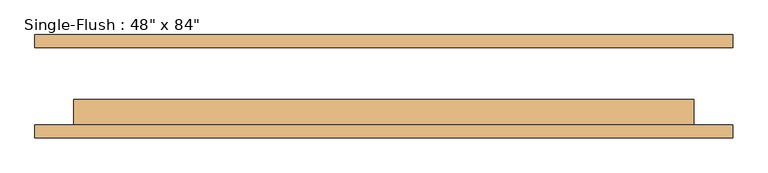
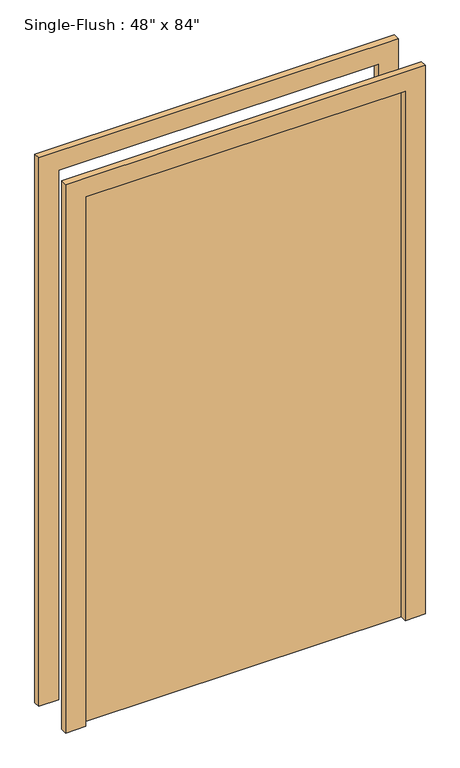
"""IFC4 building model written with IfcOpenShell, lengths in millimetres: door geometry."""

from ifc_helpers import new_model, si_unit, frame, origin, origin_with_axes, place, context, project, spatial, polyline, outline, extrude, source, transform, mapped, element, save


def door_3737b4f8(model_context):
    return source(origin(), model_context, "Body", "SweptSolid", [
        extrude(outline(polyline([(2209.8, -685.8), (0.0, -685.8), (0.0, -609.6), (2133.6, -609.6), (2133.6, 609.6), (0.0, 609.6), (0.0, 685.8), (2209.8, 685.8), (2209.8, -685.8)])), frame((0.0, -101.6, 0.0), z_axis=(0.0, 1.0, 0.0), x_axis=(0.0, 0.0, 1.0)), (0.0, 0.0, 1.0), 25.4),
        extrude(outline(polyline([(2209.8, 685.8), (2209.8, -685.8), (0.0, -685.8), (0.0, -609.6), (2133.6, -609.6), (2133.6, 609.6), (0.0, 609.6), (0.0, 685.8), (2209.8, 685.8)])), frame((0.0, 76.2, 0.0), z_axis=(0.0, 1.0, 0.0), x_axis=(0.0, 0.0, 1.0)), (0.0, 0.0, 1.0), 25.4),
        extrude(outline(polyline([(609.6, -25.4), (609.6, -76.2), (-609.6, -76.2), (-609.6, -25.4), (609.6, -25.4)])), origin_with_axes(), (0.0, 0.0, 1.0), 2133.6),
    ])


if __name__ == "__main__":
    model = new_model("IFC4")
    model_context = context("Model", 3, world=origin())
    ifc_project = project(units=[si_unit("LENGTHUNIT", "METRE", prefix="MILLI")], contexts=[model_context])
    site = spatial("IfcSite", under=ifc_project)
    building = spatial("IfcBuilding", under=site)
    placement = place(None, origin())
    door_shape = door_3737b4f8(model_context)
    element("IfcDoor", 1, ObjectType="Single-Flush : 48\" x 84\"", at=placement, inside=building, context=model_context, shape_type="MappedRepresentation", body=[
        mapped(door_shape, transform((0.0, 0.0, 0.0), x_axis=(1.0, 0.0, 0.0), y_axis=(0.0, 1.0, 0.0), z_axis=(0.0, 0.0, 1.0))),
    ])
    save(model, "model.ifc")

# Revit data of these elements
# Type "Single-Flush : 48\" x 84\""
#   Type Mark = "8"
#   Construction Type Id = "MDOOR"
#   Assembly Code = "C1020"
#   Analytic Construction = "Metal"
#   Thickness = 0' - 2"
#   Heat Transfer Coefficient (U) = 0.651978 BTU/(h·ft²·°F)
#   Height = 7' - 0"
#   Trim Projection Ext = 0' - 1"
#   Trim Projection Int = 0' - 1"
#   Trim Width = 0' - 3"
#   Width = 4' - 0"
#   Define Thermal Properties by = 1
#   Door Material = Door - Panel
#   Frame Material = Door - Frame
#   Visual Light Transmittance = 0
#   Solar Heat Gain Coefficient = 0
#   Function = (empty or 0)
#   Wall Closure = (empty or 0)
# Element 1 (IfcDoor, "Single-Flush : 48\" x 84\"")
#   Materials on its faces: "Door - Frame", "Door - Panel"
# Materials
#   "Door - Panel": class "Wood", colour RGB 210 159 95, transparency 0, Cost = 0
#   "Door - Frame": colour RGB 118 70 51, transparency 0, Cost = 0
